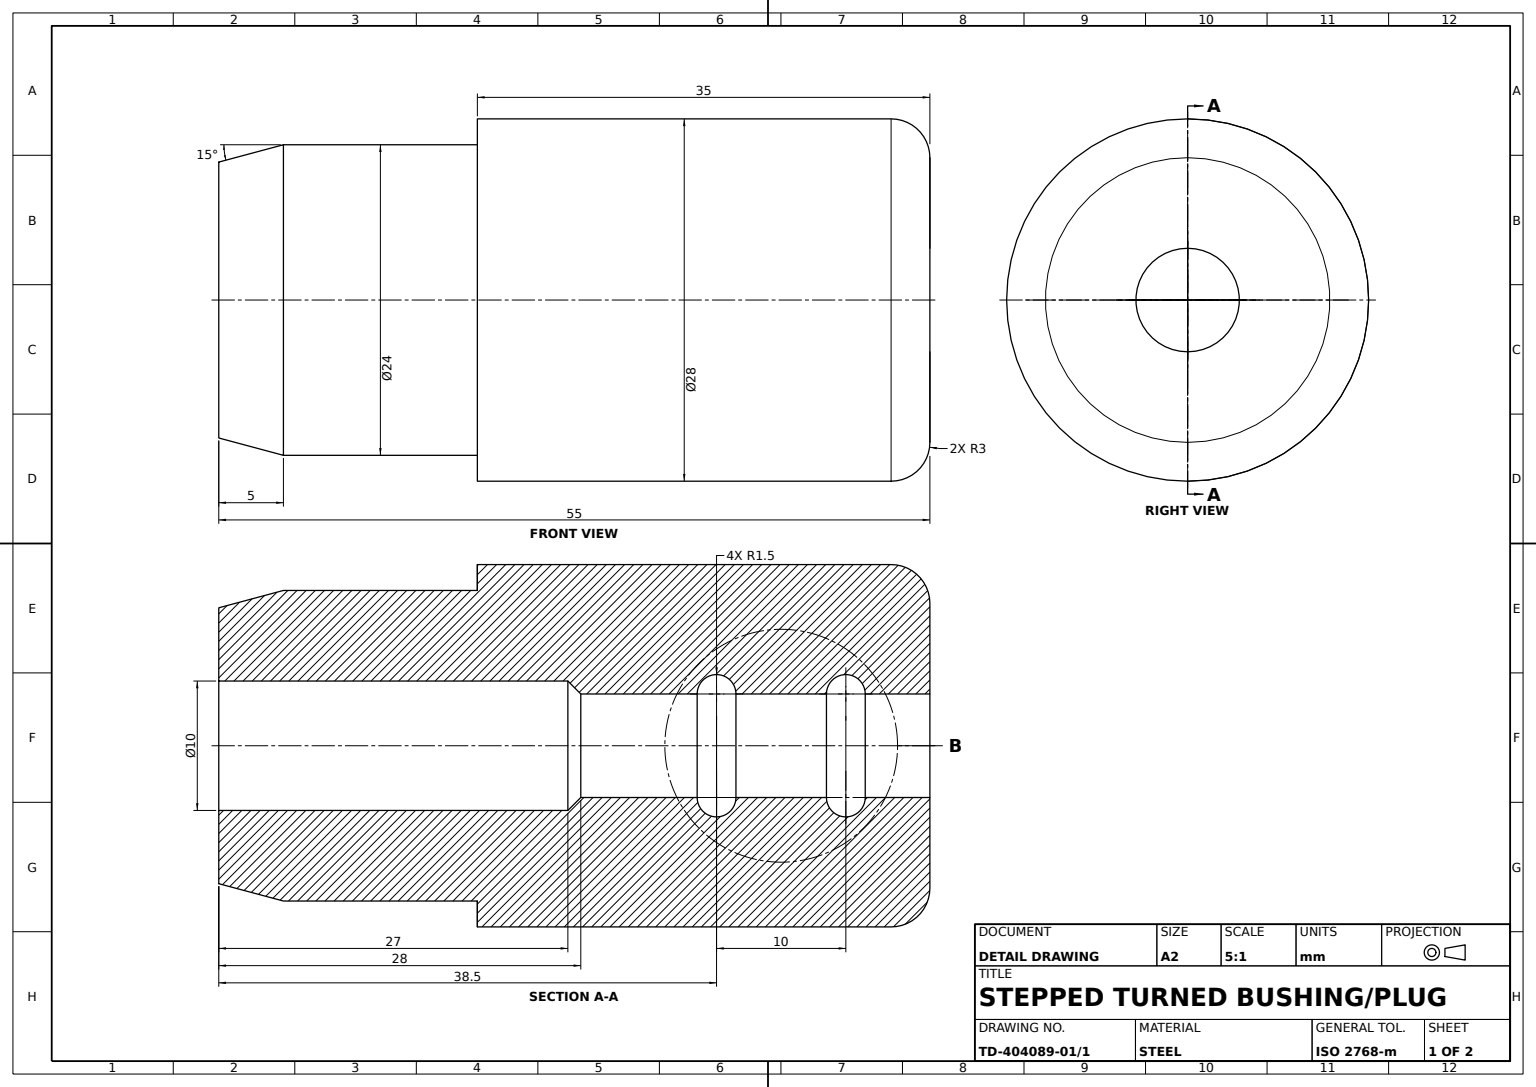
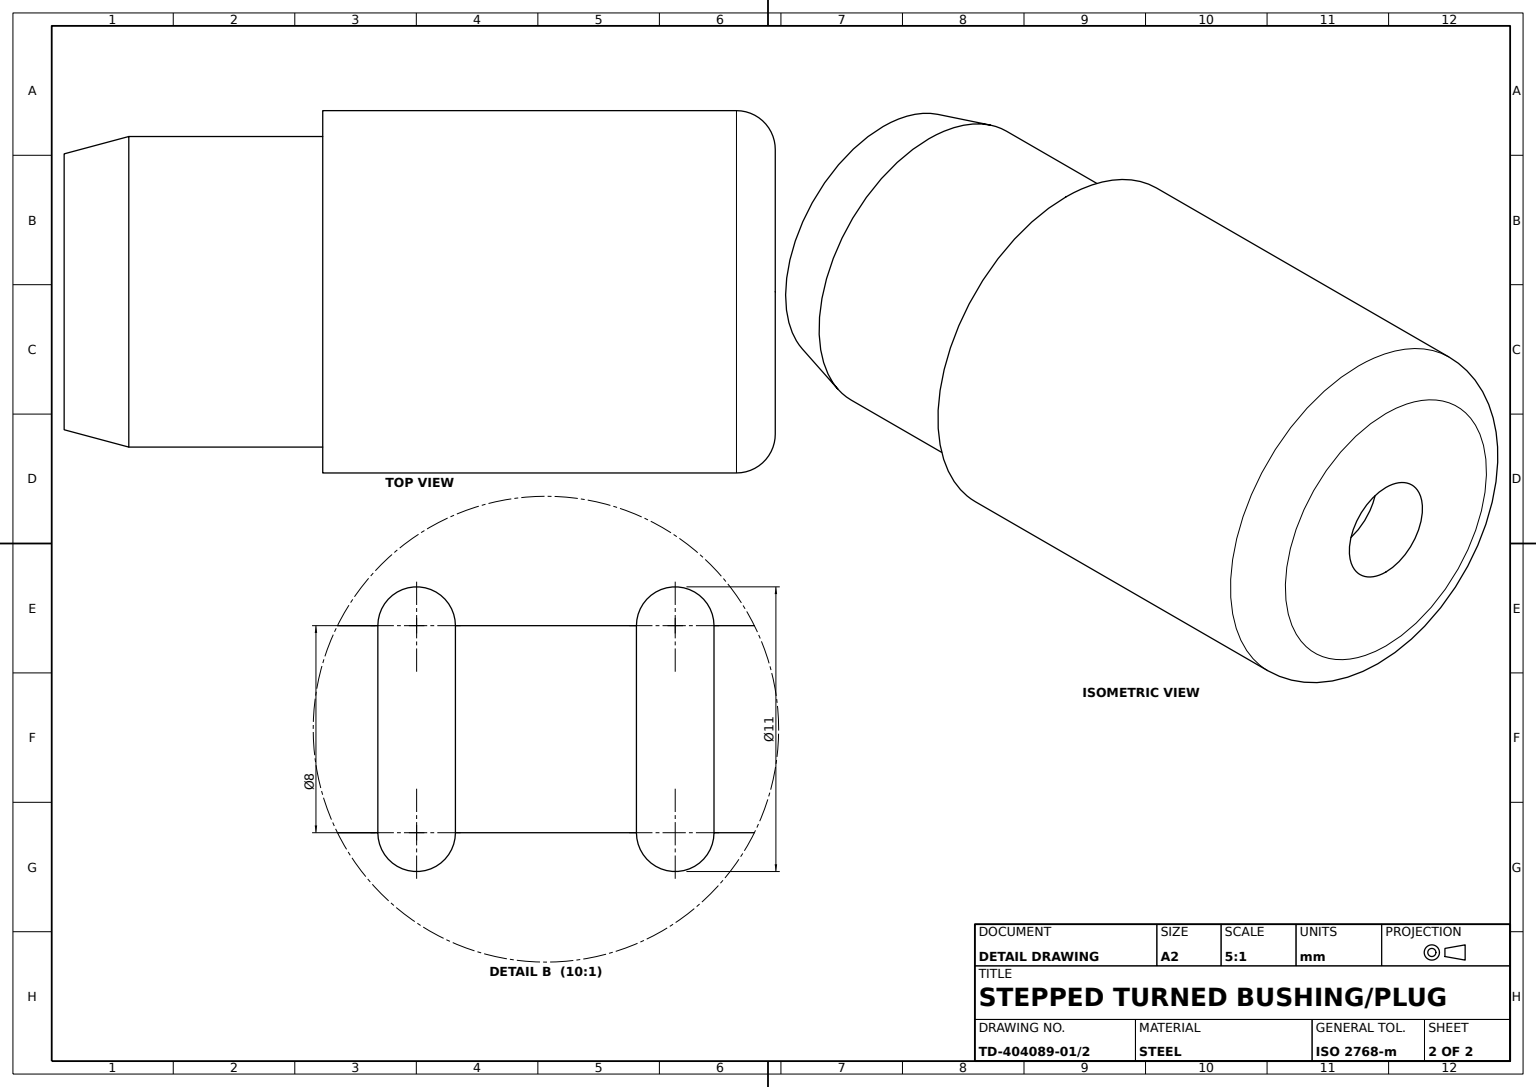
from build123d import *


with BuildPart() as part:
    # Pin Revolve Profile → Pin Body Revolve (revolve)
    with BuildSketch(Plane.XY):
        with BuildLine():
            Line((-4, 60.189864048), (-4, 65.189864048))
            Line((-4, 65.189864048), (-11, 65.189864048))
            ThreePointArc((-11, 65.189864048), (-13.121320344, 64.311184392), (-14, 62.189864048))
            Line((-14, 62.189864048), (-14, 30.189864048))
            Line((-14, 30.189864048), (-12, 30.189864048))
            Line((-12, 30.189864048), (-12, 15.189864048))
            Line((-12, 15.189864048), (-10.660254038, 10.189864048))
            Line((-10.660254038, 10.189864048), (-5, 10.189864048))
            Line((-5, 10.189864048), (-5, 37.189864048))
            Line((-5, 37.189864048), (-4, 38.189864048))
            Line((-4, 38.189864048), (-4, 47.189864048))
            ThreePointArc((-4, 47.189864048), (-5.5, 48.689864048), (-4, 50.189864048))
            Line((-4, 50.189864048), (-4, 57.189864048))
            ThreePointArc((-4, 57.189864048), (-5.5, 58.689864048), (-4, 60.189864048))
        make_face()
    revolve(axis=Axis((0, 148.451497923, 0), (0, -1, 0)))


solid = part.part
